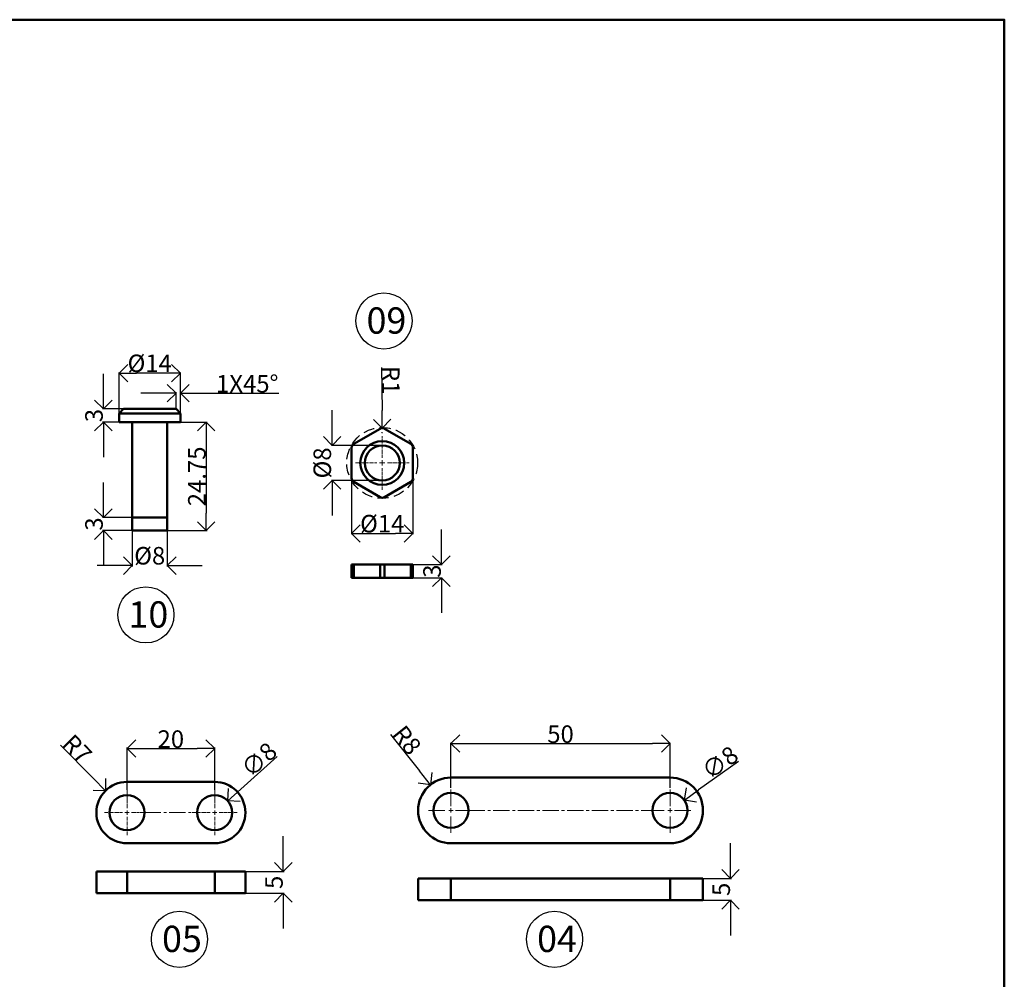
# Model space of a CAD drawing. Units: millimetres. Extents: x 45 to 546, y 51 to 638.
# Tile 4 of 4: x 322 to 546, y 419 to 638. Entities that reach past the tile are written whole.
import ezdxf

# ---------------------------------------------------------------- set-up
doc = ezdxf.new("R2010")
doc.units = ezdxf.units.MM
doc.header["$MEASUREMENT"] = 0
doc.linetypes.add('CENTER2', pattern=[1.125, 0.75, -0.125, 0.125, -0.125])
doc.linetypes.add('HIDDEN', pattern=[0.375, 0.25, -0.125])
for name, color, linetype, lineweight in [('M-CNTR', 1, 'CENTER2', 18), ('M-DIMS', 2, 'Continuous', 25), ('M-HIDN', 8, 'HIDDEN', 25), ('M-OUTL', 7, 'Continuous', 50), ('M-TEXT', 7, 'Continuous', 25), ('M-TTLB', 7, 'Continuous', 50)]:
    doc.layers.add(name, color=color, linetype=linetype, lineweight=lineweight)
doc.styles.get("Standard").update_dxf_attribs({"font": 'arial.ttf'})
doc.dimstyles.get("Standard").update_dxf_attribs({"dimtxt": 4, "dimasz": 4, "dimexe": 0.18, "dimexo": 0.0625, "dimgap": 0.09, "dimtad": 1, "dimdec": 0, "dimzin": 0, "dimdsep": 46, "dimtxsty": 'Standard', "dimblk": 'OPEN90', "dimcen": 0.09, "dimclre": 251, "dimadec": 0, "dimazin": 0, "dimtfac": 1, "dimtdec": 0, "dimtofl": 0, "dimtmove": 0, "dimatfit": 3, "dimfxl": 1, "dimtolj": 1, "dimtzin": 0, "dimarcsym": 0})

# ---------------------------------------------------------------- blocks, each defined once
blk = doc.blocks.new('_Open90')
at = {"color": 0, "linetype": 'ByBlock', "lineweight": -2}
for p, q in [((0, 0), (-1, 0)), ((-0.5, 0.5), (0, 0)), ((0, 0), (-0.5, -0.5))]:
    blk.add_line(p, q, dxfattribs=at)
blk = doc.blocks.new('*D31')
at = {"layer": 'Defpoints', "color": 0, "transparency": 16777216}
for p in [(358.26, 546.08), (355.26, 521.33), (364.15, 521.33)]:
    blk.add_point(p, dxfattribs=at)
at = {"layer": 'M-DIMS', "color": 0, "lineweight": -2, "transparency": 16777216}
for p, q in [((358.33, 546.08), (364.33, 546.08)), ((364.15, 542.08), (364.15, 525.33)), ((355.33, 521.33), (364.33, 521.33))]:
    blk.add_line(p, q, dxfattribs=at)
at = {"layer": 'M-DIMS', "color": 0, "lineweight": -2, "transparency": 16777216, "xscale": 4, "yscale": 4, "zscale": 4}
for p, rotation in [((364.15, 546.08), 90), ((364.15, 521.33), 270)]:
    blk.add_blockref('_Open90', p, dxfattribs=dict(at, rotation=rotation))
at = {"layer": 'M-DIMS', "color": 0, "transparency": 16777216, "insert": (362.01, 533.7), "char_height": 4, "attachment_point": 5, "rotation": 90}
blk.add_mtext('\\A1;24.75', dxfattribs=at)
blk = doc.blocks.new('*D32')
at = {"layer": 'Defpoints', "color": 0, "transparency": 16777216}
for p in [(344.26, 557.25), (344.26, 548.08), (358.26, 548.08)]:
    blk.add_point(p, dxfattribs=at)
at = {"layer": 'M-DIMS', "color": 0, "lineweight": -2, "transparency": 16777216}
for p, q in [((344.26, 548.14), (344.26, 557.43)), ((354.26, 557.25), (348.26, 557.25)), ((358.26, 548.14), (358.26, 557.43))]:
    blk.add_line(p, q, dxfattribs=at)
at = {"layer": 'M-DIMS', "color": 0, "lineweight": -2, "transparency": 16777216, "xscale": 4, "yscale": 4, "zscale": 4, "rotation": 180}
blk.add_blockref('_Open90', (344.26, 557.25), dxfattribs=at)
at = {"layer": 'M-DIMS', "color": 0, "lineweight": -2, "transparency": 16777216, "xscale": 4, "yscale": 4, "zscale": 4}
blk.add_blockref('_Open90', (358.26, 557.25), dxfattribs=at)
at = {"layer": 'M-DIMS', "color": 0, "transparency": 16777216, "insert": (351.26, 559.5), "char_height": 4, "attachment_point": 5}
blk.add_mtext('\\A1;%%C14', dxfattribs=at)
blk = doc.blocks.new('*D33')
at = {"layer": 'Defpoints', "color": 0, "transparency": 16777216}
for p in [(340.68, 549.08), (345.26, 549.08), (344.26, 546.08)]:
    blk.add_point(p, dxfattribs=at)
at = {"layer": 'M-DIMS', "color": 0, "lineweight": -2, "transparency": 16777216}
for p, q in [((340.68, 553.08), (340.68, 557.08)), ((345.2, 549.08), (340.5, 549.08)), ((344.2, 546.08), (340.5, 546.08)), ((340.68, 542.08), (340.68, 538.08))]:
    blk.add_line(p, q, dxfattribs=at)
at = {"layer": 'M-DIMS', "color": 0, "lineweight": -2, "transparency": 16777216, "xscale": 4, "yscale": 4, "zscale": 4}
for p, rotation in [((340.68, 549.08), 270), ((340.68, 546.08), 90)]:
    blk.add_blockref('_Open90', p, dxfattribs=dict(at, rotation=rotation))
at = {"layer": 'M-DIMS', "color": 0, "transparency": 16777216, "insert": (338.55, 547.58), "char_height": 4, "attachment_point": 5, "rotation": 90}
blk.add_mtext('\\A1;3', dxfattribs=at)
blk = doc.blocks.new('*D34')
at = {"layer": 'Defpoints', "color": 0, "transparency": 16777216}
for p in [(340.68, 524.33), (347.26, 524.33), (347.26, 521.33)]:
    blk.add_point(p, dxfattribs=at)
at = {"layer": 'M-DIMS', "color": 0, "lineweight": -2, "transparency": 16777216}
for p, q in [((340.68, 528.33), (340.68, 532.33)), ((347.2, 524.33), (340.5, 524.33)), ((347.2, 521.33), (340.5, 521.33)), ((340.68, 517.33), (340.68, 513.33))]:
    blk.add_line(p, q, dxfattribs=at)
at = {"layer": 'M-DIMS', "color": 0, "lineweight": -2, "transparency": 16777216, "xscale": 4, "yscale": 4, "zscale": 4}
for p, rotation in [((340.68, 524.33), 270), ((340.68, 521.33), 90)]:
    blk.add_blockref('_Open90', p, dxfattribs=dict(at, rotation=rotation))
at = {"layer": 'M-DIMS', "color": 0, "transparency": 16777216, "insert": (338.55, 522.83), "char_height": 4, "attachment_point": 5, "rotation": 90}
blk.add_mtext('\\A1;3', dxfattribs=at)
blk = doc.blocks.new('*D35')
at = {"layer": 'Defpoints', "color": 0, "transparency": 16777216}
for p in [(347.26, 521.33), (355.26, 521.33), (347.26, 513.34)]:
    blk.add_point(p, dxfattribs=at)
at = {"layer": 'M-DIMS', "color": 0, "lineweight": -2, "transparency": 16777216}
for p, q in [((347.26, 521.26), (347.26, 513.16)), ((355.26, 521.26), (355.26, 513.16)), ((343.26, 513.34), (339.26, 513.34)), ((359.26, 513.34), (363.26, 513.34))]:
    blk.add_line(p, q, dxfattribs=at)
at = {"layer": 'M-DIMS', "color": 0, "lineweight": -2, "transparency": 16777216, "xscale": 4, "yscale": 4, "zscale": 4}
blk.add_blockref('_Open90', (347.26, 513.34), dxfattribs=at)
at = {"layer": 'M-DIMS', "color": 0, "lineweight": -2, "transparency": 16777216, "xscale": 4, "yscale": 4, "zscale": 4, "rotation": 180}
blk.add_blockref('_Open90', (355.26, 513.34), dxfattribs=at)
at = {"layer": 'M-DIMS', "color": 0, "transparency": 16777216, "insert": (351.26, 515.59), "char_height": 4, "attachment_point": 5}
blk.add_mtext('\\A1;%%C8', dxfattribs=at)
blk = doc.blocks.new('*D36')
at = {"layer": 'Defpoints', "color": 0, "transparency": 16777216}
for p in [(358.26, 552.7), (357.26, 549.08), (358.26, 548.08)]:
    blk.add_point(p, dxfattribs=at)
at = {"layer": 'M-DIMS', "color": 0, "lineweight": -2, "transparency": 16777216}
for p, q in [((353.26, 552.7), (349.26, 552.7)), ((357.26, 549.14), (357.26, 552.88)), ((358.26, 548.14), (358.26, 552.88)), ((362.26, 552.7), (380.75, 552.7))]:
    blk.add_line(p, q, dxfattribs=at)
at = {"layer": 'M-DIMS', "color": 0, "lineweight": -2, "transparency": 16777216, "xscale": 4, "yscale": 4, "zscale": 4}
blk.add_blockref('_Open90', (357.26, 552.7), dxfattribs=at)
at = {"layer": 'M-DIMS', "color": 0, "lineweight": -2, "transparency": 16777216, "xscale": 4, "yscale": 4, "zscale": 4, "rotation": 180}
blk.add_blockref('_Open90', (358.26, 552.7), dxfattribs=at)
at = {"layer": 'M-DIMS', "color": 0, "transparency": 16777216, "insert": (373.51, 554.83), "char_height": 4, "attachment_point": 5}
blk.add_mtext('\\A1;1X45%%D', dxfattribs=at)
blk = doc.blocks.new('*U37')
at = {"layer": 'M-CNTR', "color": 0, "transparency": 16777216}
for p, q in [((0, 1.2), (0, 6.12)), ((-6.12, 0), (-1.2, 0)), ((1.2, 0), (6.12, 0)), ((0, -6.12), (0, -1.2))]:
    blk.add_line(p, q, dxfattribs=at)
at = {"layer": 'M-CNTR', "color": 0, "linetype": 'Continuous', "transparency": 16777216}
for p, q in [((-0.6, 0), (0.6, 0)), ((0, -0.6), (0, 0.6))]:
    blk.add_line(p, q, dxfattribs=at)
blk = doc.blocks.new('*D38')
at = {"layer": 'Defpoints', "color": 0, "transparency": 16777216}
for p in [(397.31, 534.04), (411.31, 532.73), (411.31, 520.67)]:
    blk.add_point(p, dxfattribs=at)
at = {"layer": 'M-DIMS', "color": 0, "lineweight": -2, "transparency": 16777216}
for p, q in [((397.31, 533.98), (397.31, 520.49)), ((411.31, 532.66), (411.31, 520.49)), ((401.31, 520.67), (407.31, 520.67))]:
    blk.add_line(p, q, dxfattribs=at)
at = {"layer": 'M-DIMS', "color": 0, "lineweight": -2, "transparency": 16777216, "xscale": 4, "yscale": 4, "zscale": 4, "rotation": 180}
blk.add_blockref('_Open90', (397.31, 520.67), dxfattribs=at)
at = {"layer": 'M-DIMS', "color": 0, "lineweight": -2, "transparency": 16777216, "xscale": 4, "yscale": 4, "zscale": 4}
blk.add_blockref('_Open90', (411.31, 520.67), dxfattribs=at)
at = {"layer": 'M-DIMS', "color": 0, "transparency": 16777216, "insert": (404.31, 522.91), "char_height": 4, "attachment_point": 5}
blk.add_mtext('\\A1;%%C14', dxfattribs=at)
blk = doc.blocks.new('*D39')
at = {"layer": 'Defpoints', "color": 0, "transparency": 16777216}
for p in [(392.88, 540.77), (404.31, 540.77), (404.31, 532.77)]:
    blk.add_point(p, dxfattribs=at)
at = {"layer": 'M-DIMS', "color": 0, "lineweight": -2, "transparency": 16777216}
for p, q in [((392.88, 544.77), (392.88, 548.77)), ((404.24, 540.77), (392.7, 540.77)), ((404.24, 532.77), (392.7, 532.77)), ((392.88, 528.77), (392.88, 524.77))]:
    blk.add_line(p, q, dxfattribs=at)
at = {"layer": 'M-DIMS', "color": 0, "lineweight": -2, "transparency": 16777216, "xscale": 4, "yscale": 4, "zscale": 4}
for p, rotation in [((392.88, 540.77), 270), ((392.88, 532.77), 90)]:
    blk.add_blockref('_Open90', p, dxfattribs=dict(at, rotation=rotation))
at = {"layer": 'M-DIMS', "color": 0, "transparency": 16777216, "insert": (390.63, 536.77), "char_height": 4, "attachment_point": 5, "rotation": 90}
blk.add_mtext('\\A1;%%C8', dxfattribs=at)
blk = doc.blocks.new('*D40')
at = {"layer": 'Defpoints', "color": 0, "transparency": 16777216}
for p in [(404.3, 544.7), (404.31, 543.7)]:
    blk.add_point(p, dxfattribs=at)
at = {"layer": 'M-DIMS', "color": 0, "lineweight": -2, "transparency": 16777216}
for p, q in [((404.16, 558.55), (404.26, 548.7)), ((404.22, 543.7), (404.4, 543.7)), ((404.31, 543.61), (404.31, 543.79))]:
    blk.add_line(p, q, dxfattribs=at)
at = {"layer": 'M-DIMS', "color": 0, "lineweight": -2, "transparency": 16777216, "xscale": 4, "yscale": 4, "zscale": 4, "rotation": 270.5525065615556}
blk.add_blockref('_Open90', (404.3, 544.7), dxfattribs=at)
at = {"layer": 'M-DIMS', "color": 0, "transparency": 16777216, "insert": (406.29, 555.64), "char_height": 4, "attachment_point": 5, "rotation": 270.5525}
blk.add_mtext('\\A1;R1', dxfattribs=at)
blk = doc.blocks.new('*D41')
at = {"layer": 'Defpoints', "color": 0, "transparency": 16777216}
for p in [(411.31, 513.58), (411.31, 510.58), (417.81, 510.58)]:
    blk.add_point(p, dxfattribs=at)
at = {"layer": 'M-DIMS', "color": 0, "lineweight": -2, "transparency": 16777216}
for p, q in [((417.81, 517.58), (417.81, 521.58)), ((411.37, 513.58), (417.99, 513.58)), ((411.37, 510.58), (417.99, 510.58)), ((417.81, 506.58), (417.81, 502.58))]:
    blk.add_line(p, q, dxfattribs=at)
at = {"layer": 'M-DIMS', "color": 0, "lineweight": -2, "transparency": 16777216, "xscale": 4, "yscale": 4, "zscale": 4}
for p, rotation in [((417.81, 513.58), 270), ((417.81, 510.58), 90)]:
    blk.add_blockref('_Open90', p, dxfattribs=dict(at, rotation=rotation))
at = {"layer": 'M-DIMS', "color": 0, "transparency": 16777216, "insert": (415.67, 512.08), "char_height": 4, "attachment_point": 5, "rotation": 90}
blk.add_mtext('\\A1;3', dxfattribs=at)
blk = doc.blocks.new('*U42')
at = {"layer": 'M-CNTR', "color": 0, "transparency": 16777216}
for p, q in [((0, 1), (0, 5.12)), ((-5.12, 0), (-1, 0)), ((1, 0), (5.12, 0)), ((0, -5.12), (0, -1))]:
    blk.add_line(p, q, dxfattribs=at)
at = {"layer": 'M-CNTR', "color": 0, "linetype": 'Continuous', "transparency": 16777216}
for p, q in [((-0.5, 0), (0.5, 0)), ((0, -0.5), (0, 0.5))]:
    blk.add_line(p, q, dxfattribs=at)
blk = doc.blocks.new('*U43')
at = {"layer": 'M-CNTR', "color": 0, "transparency": 16777216}
for p, q in [((0, 1), (0, 5.12)), ((-5.12, 0), (-1, 0)), ((1, 0), (5.12, 0)), ((0, -5.12), (0, -1))]:
    blk.add_line(p, q, dxfattribs=at)
at = {"layer": 'M-CNTR', "color": 0, "linetype": 'Continuous', "transparency": 16777216}
for p, q in [((-0.5, 0), (0.5, 0)), ((0, -0.5), (0, 0.5))]:
    blk.add_line(p, q, dxfattribs=at)
blk = doc.blocks.new('*D44')
at = {"layer": 'Defpoints', "color": 0, "transparency": 16777216}
for p in [(341.17, 461.98), (346.08, 457)]:
    blk.add_point(p, dxfattribs=at)
at = {"layer": 'M-DIMS', "color": 0, "lineweight": -2, "transparency": 16777216}
for p, q in [((330.91, 472.41), (338.37, 464.84)), ((345.99, 457), (346.17, 457)), ((346.08, 456.91), (346.08, 457.09))]:
    blk.add_line(p, q, dxfattribs=at)
at = {"layer": 'M-DIMS', "color": 0, "lineweight": -2, "transparency": 16777216, "xscale": 4, "yscale": 4, "zscale": 4, "rotation": 314.5387038348235}
blk.add_blockref('_Open90', (341.17, 461.98), dxfattribs=at)
at = {"layer": 'M-DIMS', "color": 0, "transparency": 16777216, "insert": (334.73, 471.52), "char_height": 4, "attachment_point": 5, "rotation": 314.5387}
blk.add_mtext('\\A1;R7', dxfattribs=at)
blk = doc.blocks.new('*D45')
at = {"layer": 'Defpoints', "color": 0, "transparency": 16777216}
for p in [(366.08, 471.63), (346.08, 462.12), (366.08, 462.12)]:
    blk.add_point(p, dxfattribs=at)
at = {"layer": 'M-DIMS', "color": 0, "lineweight": -2, "transparency": 16777216}
for p, q in [((346.08, 462.18), (346.08, 471.81)), ((366.08, 462.18), (366.08, 471.81)), ((350.08, 471.63), (362.08, 471.63))]:
    blk.add_line(p, q, dxfattribs=at)
at = {"layer": 'M-DIMS', "color": 0, "lineweight": -2, "transparency": 16777216, "xscale": 4, "yscale": 4, "zscale": 4, "rotation": 180}
blk.add_blockref('_Open90', (346.08, 471.63), dxfattribs=at)
at = {"layer": 'M-DIMS', "color": 0, "lineweight": -2, "transparency": 16777216, "xscale": 4, "yscale": 4, "zscale": 4}
blk.add_blockref('_Open90', (366.08, 471.63), dxfattribs=at)
at = {"layer": 'M-DIMS', "color": 0, "transparency": 16777216, "insert": (356.08, 473.76), "char_height": 4, "attachment_point": 5}
blk.add_mtext('\\A1;20', dxfattribs=at)
blk = doc.blocks.new('*D46')
at = {"layer": 'Defpoints', "color": 0, "transparency": 16777216}
for p in [(369.06, 459.66), (363.1, 454.33)]:
    blk.add_point(p, dxfattribs=at)
at = {"layer": 'M-DIMS', "color": 0, "lineweight": -2, "transparency": 16777216}
for p, q in [((380.36, 469.78), (372.04, 462.33)), ((365.99, 457), (366.17, 457)), ((366.08, 456.91), (366.08, 457.09))]:
    blk.add_line(p, q, dxfattribs=at)
at = {"layer": 'M-DIMS', "color": 0, "lineweight": -2, "transparency": 16777216, "xscale": 4, "yscale": 4, "zscale": 4, "rotation": 221.8399971371856}
blk.add_blockref('_Open90', (369.06, 459.66), dxfattribs=at)
at = {"layer": 'M-DIMS', "color": 0, "transparency": 16777216, "insert": (376.19, 469.06), "char_height": 4, "attachment_point": 5, "rotation": 41.84}
blk.add_mtext('\\A1;∅8', dxfattribs=at)
blk = doc.blocks.new('*D47')
at = {"layer": 'Defpoints', "color": 0, "transparency": 16777216}
for p in [(373.08, 443.58), (373.08, 438.58), (381.73, 438.58)]:
    blk.add_point(p, dxfattribs=at)
at = {"layer": 'M-DIMS', "color": 0, "lineweight": -2, "transparency": 16777216}
for p, q in [((381.73, 447.58), (381.73, 451.58)), ((373.15, 443.58), (381.91, 443.58)), ((373.15, 438.58), (381.91, 438.58)), ((381.73, 434.58), (381.73, 430.58))]:
    blk.add_line(p, q, dxfattribs=at)
at = {"layer": 'M-DIMS', "color": 0, "lineweight": -2, "transparency": 16777216, "xscale": 4, "yscale": 4, "zscale": 4}
for p, rotation in [((381.73, 443.58), 270), ((381.73, 438.58), 90)]:
    blk.add_blockref('_Open90', p, dxfattribs=dict(at, rotation=rotation))
at = {"layer": 'M-DIMS', "color": 0, "transparency": 16777216, "insert": (379.61, 441.08), "char_height": 4, "attachment_point": 5, "rotation": 90}
blk.add_mtext('\\A1;5', dxfattribs=at)
blk = doc.blocks.new('*U48')
at = {"layer": 'M-CNTR', "color": 0, "ltscale": 5, "transparency": 16777216}
for p, q in [((0, 1), (0, 5.12)), ((-5.12, 0), (-1, 0)), ((1, 0), (5.12, 0)), ((0, -5.12), (0, -1))]:
    blk.add_line(p, q, dxfattribs=at)
at = {"layer": 'M-CNTR', "color": 0, "linetype": 'Continuous', "ltscale": 5, "transparency": 16777216}
for p, q in [((-0.5, 0), (0.5, 0)), ((0, -0.5), (0, 0.5))]:
    blk.add_line(p, q, dxfattribs=at)
blk = doc.blocks.new('*U49')
at = {"layer": 'M-CNTR', "color": 0, "ltscale": 5, "transparency": 16777216}
for p, q in [((0, 1), (0, 5.12)), ((-5.12, 0), (-1, 0)), ((1, 0), (5.12, 0)), ((0, -5.12), (0, -1))]:
    blk.add_line(p, q, dxfattribs=at)
at = {"layer": 'M-CNTR', "color": 0, "linetype": 'Continuous', "ltscale": 5, "transparency": 16777216}
for p, q in [((-0.5, 0), (0.5, 0)), ((0, -0.5), (0, 0.5))]:
    blk.add_line(p, q, dxfattribs=at)
blk = doc.blocks.new('*D50')
at = {"layer": 'Defpoints', "color": 0, "transparency": 16777216}
for p in [(415.32, 463.36), (419.99, 457.49)]:
    blk.add_point(p, dxfattribs=at)
at = {"layer": 'M-DIMS', "color": 0, "lineweight": -2, "transparency": 16777216}
for p, q in [((406.21, 474.81), (412.83, 466.49)), ((419.9, 457.49), (420.08, 457.49)), ((419.99, 457.4), (419.99, 457.58))]:
    blk.add_line(p, q, dxfattribs=at)
at = {"layer": 'M-DIMS', "color": 0, "lineweight": -2, "transparency": 16777216, "xscale": 4, "yscale": 4, "zscale": 4, "rotation": 308.5169430426345}
blk.add_blockref('_Open90', (415.32, 463.36), dxfattribs=at)
at = {"layer": 'M-DIMS', "color": 0, "transparency": 16777216, "insert": (409.94, 473.54), "char_height": 4, "attachment_point": 5, "rotation": 308.5169}
blk.add_mtext('\\A1;R8', dxfattribs=at)
blk = doc.blocks.new('*D51')
at = {"layer": 'Defpoints', "color": 0, "transparency": 16777216}
for p in [(473.24, 459.82), (466.74, 455.16)]:
    blk.add_point(p, dxfattribs=at)
at = {"layer": 'M-DIMS', "color": 0, "lineweight": -2, "transparency": 16777216}
for p, q in [((485.57, 468.65), (476.5, 462.15)), ((469.9, 457.49), (470.08, 457.49)), ((469.99, 457.4), (469.99, 457.58))]:
    blk.add_line(p, q, dxfattribs=at)
at = {"layer": 'M-DIMS', "color": 0, "lineweight": -2, "transparency": 16777216, "xscale": 4, "yscale": 4, "zscale": 4, "rotation": 215.5957458308631}
blk.add_blockref('_Open90', (473.24, 459.82), dxfattribs=at)
at = {"layer": 'M-DIMS', "color": 0, "transparency": 16777216, "insert": (481.36, 468.39), "char_height": 4, "attachment_point": 5, "rotation": 35.5957}
blk.add_mtext('\\A1;∅8', dxfattribs=at)
blk = doc.blocks.new('*D52')
at = {"layer": 'Defpoints', "color": 0, "transparency": 16777216}
for p in [(469.99, 472.76), (419.99, 462.61), (469.99, 462.61)]:
    blk.add_point(p, dxfattribs=at)
at = {"layer": 'M-DIMS', "color": 0, "lineweight": -2, "transparency": 16777216}
for p, q in [((419.99, 462.67), (419.99, 472.94)), ((423.99, 472.76), (465.99, 472.76)), ((469.99, 462.67), (469.99, 472.94))]:
    blk.add_line(p, q, dxfattribs=at)
at = {"layer": 'M-DIMS', "color": 0, "lineweight": -2, "transparency": 16777216, "xscale": 4, "yscale": 4, "zscale": 4, "rotation": 180}
blk.add_blockref('_Open90', (419.99, 472.76), dxfattribs=at)
at = {"layer": 'M-DIMS', "color": 0, "lineweight": -2, "transparency": 16777216, "xscale": 4, "yscale": 4, "zscale": 4}
blk.add_blockref('_Open90', (469.99, 472.76), dxfattribs=at)
at = {"layer": 'M-DIMS', "color": 0, "transparency": 16777216, "insert": (444.99, 474.89), "char_height": 4, "attachment_point": 5}
blk.add_mtext('\\A1;50', dxfattribs=at)
blk = doc.blocks.new('*D53')
at = {"layer": 'Defpoints', "color": 0, "transparency": 16777216}
for p in [(477.49, 441.98), (477.49, 436.98), (483.78, 436.98)]:
    blk.add_point(p, dxfattribs=at)
at = {"layer": 'M-DIMS', "color": 0, "lineweight": -2, "transparency": 16777216}
for p, q in [((483.78, 445.98), (483.78, 449.98)), ((477.55, 441.98), (483.96, 441.98)), ((477.55, 436.98), (483.96, 436.98)), ((483.78, 432.98), (483.78, 428.98))]:
    blk.add_line(p, q, dxfattribs=at)
at = {"layer": 'M-DIMS', "color": 0, "lineweight": -2, "transparency": 16777216, "xscale": 4, "yscale": 4, "zscale": 4}
for p, rotation in [((483.78, 441.98), 270), ((483.78, 436.98), 90)]:
    blk.add_blockref('_Open90', p, dxfattribs=dict(at, rotation=rotation))
at = {"layer": 'M-DIMS', "color": 0, "transparency": 16777216, "insert": (481.65, 439.48), "char_height": 4, "attachment_point": 5, "rotation": 90}
blk.add_mtext('\\A1;5', dxfattribs=at)

msp = doc.modelspace()

# ---------------------------------------------------------------- linework, layer by layer
at = {"layer": 'M-CNTR', "ltscale": 5}
for p, q in [((350.083, 456.995), (362.083, 456.995)), ((423.992, 457.492), (465.992, 457.492))]:
    msp.add_line(p, q, dxfattribs=at)
at = {"layer": 'M-HIDN', "ltscale": 10}
msp.add_circle((404.306, 536.768), 8.083, dxfattribs=at)
at = {"layer": 'M-OUTL'}
for p, q in [((344.263, 548.077), (345.263, 549.077)), ((345.263, 549.077), (357.263, 549.077)), ((357.263, 549.077), (358.263, 548.077)), ((344.263, 548.077), (344.263, 546.077)), ((344.263, 548.077), (358.263, 548.077)), ((344.263, 546.077), (358.263, 546.077)), ((347.263, 546.077), (347.263, 521.327)), ((355.263, 546.077), (355.263, 521.327)), ((358.263, 546.077), (358.263, 548.077)), ((347.263, 524.327), (355.263, 524.327)), ((347.263, 521.327), (355.263, 521.327)), ((397.306, 510.584), (397.306, 513.584)), ((397.306, 513.584), (411.306, 513.584)), ((397.806, 510.584), (397.806, 513.584)), ((403.806, 510.584), (403.806, 513.584)), ((404.806, 510.584), (404.806, 513.584)), ((410.806, 510.584), (410.806, 513.584)), ((411.306, 510.584), (411.306, 513.584)), ((397.306, 510.584), (411.306, 510.584)), ((346.083, 463.995), (366.083, 463.995)), ((419.992, 464.992), (469.992, 464.992)), ((346.083, 449.995), (366.083, 449.995)), ((419.992, 449.992), (469.992, 449.992)), ((339.083, 438.58), (339.083, 443.58)), ((339.083, 443.58), (373.083, 443.58)), ((346.083, 443.58), (346.083, 438.58)), ((366.083, 443.58), (366.083, 438.58)), ((373.083, 438.58), (373.083, 443.58)), ((412.492, 441.977), (412.492, 436.977)), ((412.492, 441.977), (477.492, 441.977)), ((419.992, 441.977), (419.992, 436.977)), ((469.992, 441.977), (469.992, 436.977)), ((477.492, 441.977), (477.492, 436.977)), ((339.083, 438.58), (373.083, 438.58)), ((412.492, 436.977), (477.492, 436.977))]:
    msp.add_line(p, q, dxfattribs=at)
msp.add_lwpolyline([(410.806, 541.098), (404.806, 544.562, 0.2679492), (403.806, 544.562), (397.806, 541.098, 0.2679492), (397.306, 540.232), (397.306, 533.304, 0.2679492), (397.806, 532.438), (403.806, 528.973, 0.2679492), (404.806, 528.973), (410.806, 532.438, 0.2679492), (411.306, 533.304), (411.306, 540.232, 0.2679492)], format="xyb", close=True, dxfattribs=at)
for centre, radius in [((404.306, 536.768), 5), ((404.306, 536.768), 4), ((346.083, 456.995), 4), ((366.083, 456.995), 4), ((419.992, 457.492), 4), ((469.992, 457.492), 4)]:
    msp.add_circle(centre, radius, dxfattribs=at)
for centre, radius, start, end in [((346.083, 456.995), 7, 90, 270), ((366.083, 456.995), 7, 270, 90), ((419.992, 457.492), 7.5, 90, 270), ((469.992, 457.492), 7.5, 270, 90)]:
    msp.add_arc(centre, radius, start, end, dxfattribs=at)
at = {"layer": 'M-TEXT'}
for centre in [(404.708, 569.163), (350.388, 502.107), (358.048, 428.083), (443.622, 428.083)]:
    msp.add_circle(centre, 6.408, dxfattribs=at)
at = {"layer": 'M-TTLB'}
msp.add_lwpolyline([(45.357, 637.893), (546.237, 637.893), (546.237, 51.054), (45.357, 51.054)], close=True, dxfattribs=at)

# ---------------------------------------------------------------- block references
at = {"layer": 'M-CNTR'}
for name, p in [('*U37', (404.306, 536.768)), ('*U42', (346.083, 456.995)), ('*U43', (366.083, 456.995))]:
    msp.add_blockref(name, p, dxfattribs=at)
at = {"layer": 'M-CNTR', "ltscale": 5}
for name, p in [('*U48', (419.992, 457.492)), ('*U49', (469.992, 457.492))]:
    msp.add_blockref(name, p, dxfattribs=at)

# ---------------------------------------------------------------- texts
at = {"layer": 'M-TEXT', "char_height": 6, "attachment_point": 1}
for s, insert in [('09', (400.728, 572.258)), ('10', (346.409, 505.203)), ('05', (354.068, 431.179)), ('04', (439.643, 431.179))]:
    msp.add_mtext_dynamic_manual_height_columns(s, width=105.49417, gutter_width=1, heights=[0], dxfattribs=dict(at, insert=insert))

# ---------------------------------------------------------------- dimensions: what is measured, and where the dimension line sits
at = {"layer": 'M-DIMS'}
for base, p1, p2, text, picture, middle in [((344.263, 557.254), (358.263, 548.077), (344.263, 548.077), '%%C<>', '*D32', (351.263, 559.498)), ((358.263, 552.696), (357.263, 549.077), (358.263, 548.077), '<>X45%%D', '*D36', (373.506, 554.828)), ((411.306, 520.666), (397.306, 534.045), (411.306, 532.726), '%%C<>', '*D38', (404.306, 522.91)), ((347.263, 513.341), (355.263, 521.327), (347.263, 521.327), '%%C<>', '*D35', (351.263, 515.586))]:
    dim = msp.add_linear_dim(base=base, p1=p1, p2=p2, text=text, dimstyle='Standard', override={"dimclrd": 0, "dimclre": 0, "dimclrt": 0}, dxfattribs=at)
    dim.commit()
    dim.dimension.update_dxf_attribs({"geometry": picture, "text_midpoint": middle})
for center, mpoint, picture, middle in [((404.306, 543.696), (404.296, 544.696), '*D40', (406.289, 555.645)), ((419.99179, 457.49155), (415.3212, 463.35973), '*D50', (409.94057, 473.54401)), ((346.083, 456.995), (341.173, 461.985), '*D44', (334.726, 471.516))]:
    dim = msp.add_radius_dim(center=center, mpoint=mpoint, dimstyle='Standard', override={"dimclrd": 0, "dimclre": 0, "dimclrt": 0}, dxfattribs=at)
    dim.commit()
    dim.dimension.update_dxf_attribs({"geometry": picture, "text_midpoint": middle})
for base, p1, p2, override, picture, middle in [((340.679, 549.077), (344.263, 546.077), (345.263, 549.077), {"dimclrd": 0, "dimclre": 0, "dimclrt": 0}, '*D33', (338.545, 547.577)), ((364.146, 521.327), (358.263, 546.077), (355.263, 521.327), {"dimdec": 2, "dimclrd": 0, "dimclre": 0, "dimclrt": 0}, '*D31', (362.013, 533.702)), ((340.679, 524.327), (347.263, 521.327), (347.263, 524.327), {"dimclrd": 0, "dimclre": 0, "dimclrt": 0}, '*D34', (338.545, 522.827)), ((417.807, 510.584), (411.306, 513.584), (411.306, 510.584), {"dimclrd": 0, "dimclre": 0, "dimclrt": 0}, '*D41', (415.673, 512.084)), ((381.729, 438.58), (373.083, 443.58), (373.083, 438.58), {"dimclrd": 0, "dimclre": 0, "dimclrt": 0}, '*D47', (379.605, 441.08)), ((483.775, 436.977), (477.492, 441.977), (477.492, 436.977), {"dimclrd": 0, "dimclre": 0, "dimclrt": 0}, '*D53', (481.651, 439.477))]:
    dim = msp.add_linear_dim(base=base, p1=p1, p2=p2, angle=90, dimstyle='Standard', override=override, dxfattribs=at)
    dim.commit()
    dim.dimension.update_dxf_attribs({"geometry": picture, "text_midpoint": middle})
dim = msp.add_linear_dim(base=(392.876, 540.768), p1=(404.306, 532.768), p2=(404.306, 540.768), angle=90, text='%%C<>', dimstyle='Standard', override={"dimclrd": 0, "dimclre": 0, "dimclrt": 0}, dxfattribs=at)
dim.commit()
dim.dimension.update_dxf_attribs({"geometry": '*D39', "text_midpoint": (390.632, 536.768)})
for base, p1, p2, picture, middle in [((366.083, 471.629), (346.083, 462.115), (366.083, 462.115), '*D45', (356.083, 473.762)), ((469.992, 472.758), (419.992, 462.612), (469.992, 462.612), '*D52', (444.992, 474.89))]:
    dim = msp.add_linear_dim(base=base, p1=p1, p2=p2, dimstyle='Standard', override={"dimclrd": 0, "dimclre": 0, "dimclrt": 0}, dxfattribs=at)
    dim.commit()
    dim.dimension.update_dxf_attribs({"geometry": picture, "text_midpoint": middle})
for p1, p2, picture, middle in [((363.102, 454.327), (369.063, 459.663), '*D46', (376.194, 469.061)), ((466.739, 455.163), (473.244, 459.82), '*D51', (481.355, 468.386))]:
    dim = msp.add_diameter_dim_2p(p1=p1, p2=p2, dimstyle='Standard', override={"dimclrd": 0, "dimclre": 0, "dimclrt": 0}, dxfattribs=at)
    dim.commit()
    dim.dimension.update_dxf_attribs({"geometry": picture, "text_midpoint": middle})

doc.saveas('drawing.dxf')
